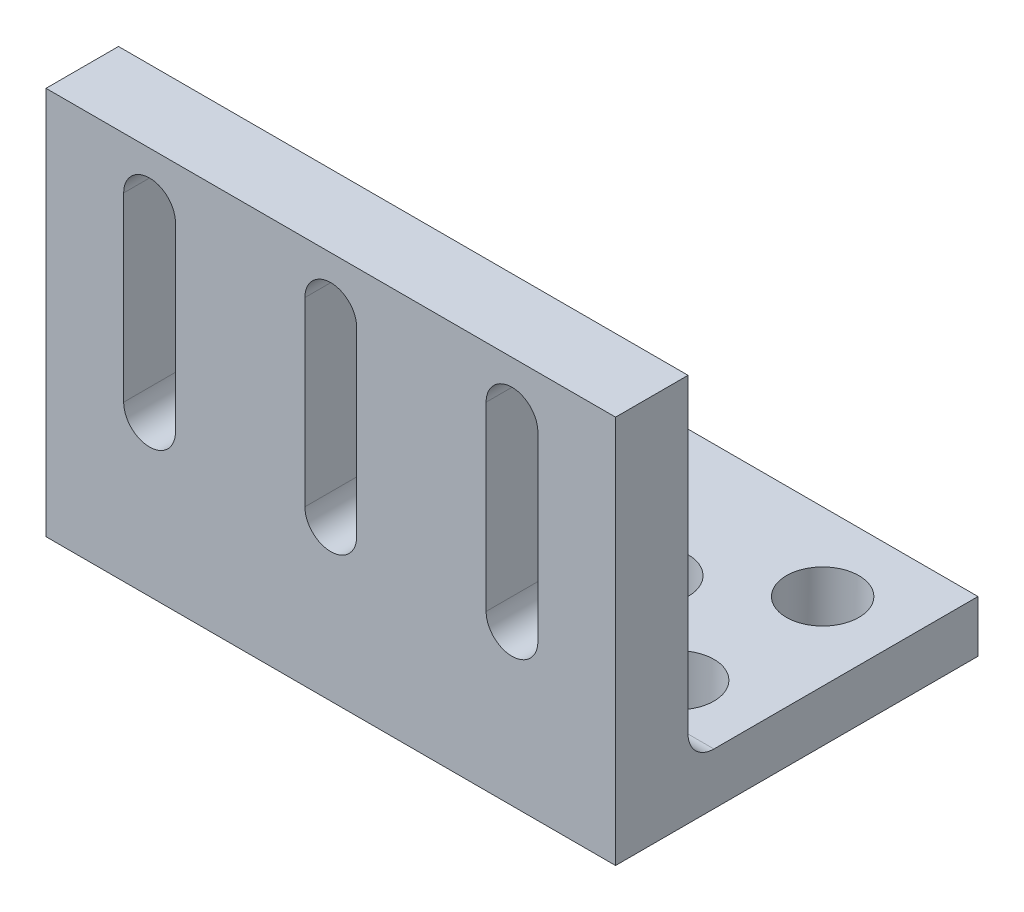
ISO-10303-21;
HEADER;
FILE_DESCRIPTION(('STEP AP214'),'2;1');
FILE_NAME('part.step','',(''),(''),'','','');
FILE_SCHEMA(('AUTOMOTIVE_DESIGN { 1 0 10303 214 1 1 1 1 }'));
ENDSEC;
DATA;
#1=APPLICATION_CONTEXT('core data for automotive mechanical design processes');
#2=APPLICATION_PROTOCOL_DEFINITION('international standard','automotive_design',2000,#1);
#3=PRODUCT_CONTEXT('',#1,'mechanical');
#4=PRODUCT('Part','Part','',(#3));
#5=PRODUCT_RELATED_PRODUCT_CATEGORY('part','',(#4));
#6=PRODUCT_DEFINITION_FORMATION('','',#4);
#7=PRODUCT_DEFINITION_CONTEXT('part definition',#1,'design');
#8=PRODUCT_DEFINITION('design','',#6,#7);
#9=PRODUCT_DEFINITION_SHAPE('','',#8);
#10=(LENGTH_UNIT() NAMED_UNIT(*) SI_UNIT(.MILLI.,.METRE.));
#11=(NAMED_UNIT(*) PLANE_ANGLE_UNIT() SI_UNIT($,.RADIAN.));
#12=(NAMED_UNIT(*) SI_UNIT($,.STERADIAN.) SOLID_ANGLE_UNIT());
#13=UNCERTAINTY_MEASURE_WITH_UNIT(LENGTH_MEASURE(1.E-05),#10,'distance_accuracy_value','');
#14=(GEOMETRIC_REPRESENTATION_CONTEXT(3) GLOBAL_UNCERTAINTY_ASSIGNED_CONTEXT((#13)) GLOBAL_UNIT_ASSIGNED_CONTEXT((#10,
#11,#12)) REPRESENTATION_CONTEXT('',''));
#15=CARTESIAN_POINT('',(0.,0.,0.));
#16=DIRECTION('',(0.,0.,1.));
#17=DIRECTION('',(1.,0.,0.));
#18=AXIS2_PLACEMENT_3D('',#15,#16,#17);
#19=CARTESIAN_POINT('',(-110.,0.,-70.));
#20=DIRECTION('',(0.,-1.,0.));
#21=DIRECTION('',(0.,0.,-1.));
#22=AXIS2_PLACEMENT_3D('',#19,#20,#21);
#23=PLANE('',#22);
#24=CARTESIAN_POINT('',(-75.,0.,-42.));
#25=DIRECTION('',(0.,-1.,0.));
#26=DIRECTION('',(0.,0.,-1.));
#27=AXIS2_PLACEMENT_3D('',#24,#25,#26);
#28=CIRCLE('',#27,7.00000000000001);
#29=CARTESIAN_POINT('',(-75.,0.,-35.));
#30=VERTEX_POINT('',#29);
#31=CARTESIAN_POINT('',(-75.,0.,-49.));
#32=VERTEX_POINT('',#31);
#33=EDGE_CURVE('E246',#30,#32,#28,.T.);
#34=ORIENTED_EDGE('',*,*,#33,.F.);
#35=DIRECTION('',(-1.,0.,0.));
#36=VECTOR('',#35,1.);
#37=CARTESIAN_POINT('',(-110.,0.,-35.));
#38=LINE('',#37,#36);
#39=CARTESIAN_POINT('',(-35.,0.,-35.));
#40=VERTEX_POINT('',#39);
#41=EDGE_CURVE('E243',#40,#30,#38,.T.);
#42=ORIENTED_EDGE('',*,*,#41,.F.);
#43=CARTESIAN_POINT('',(-35.,0.,-42.));
#44=DIRECTION('',(0.,-1.,0.));
#45=DIRECTION('',(0.,0.,-1.));
#46=AXIS2_PLACEMENT_3D('',#43,#44,#45);
#47=CIRCLE('',#46,7.);
#48=CARTESIAN_POINT('',(-35.,0.,-49.));
#49=VERTEX_POINT('',#48);
#50=EDGE_CURVE('E199',#49,#40,#47,.T.);
#51=ORIENTED_EDGE('',*,*,#50,.F.);
#52=DIRECTION('',(1.,0.,0.));
#53=VECTOR('',#52,1.);
#54=CARTESIAN_POINT('',(-110.,0.,-49.));
#55=LINE('',#54,#53);
#56=EDGE_CURVE('E249',#32,#49,#55,.T.);
#57=ORIENTED_EDGE('',*,*,#56,.F.);
#58=EDGE_LOOP('',(#34,#42,#51,#57));
#59=FACE_BOUND('',#58,.T.);
#60=CARTESIAN_POINT('',(-95.,0.,-27.));
#61=DIRECTION('',(0.,-1.,0.));
#62=DIRECTION('',(0.,0.,-1.));
#63=AXIS2_PLACEMENT_3D('',#60,#61,#62);
#64=CIRCLE('',#63,7.);
#65=CARTESIAN_POINT('',(-95.,0.,-34.));
#66=VERTEX_POINT('',#65);
#67=EDGE_CURVE('E241',#66,#66,#64,.T.);
#68=ORIENTED_EDGE('',*,*,#67,.F.);
#69=EDGE_LOOP('',(#68));
#70=FACE_BOUND('',#69,.T.);
#71=CARTESIAN_POINT('',(-15.,0.,-27.));
#72=DIRECTION('',(0.,-1.,0.));
#73=DIRECTION('',(0.,0.,-1.));
#74=AXIS2_PLACEMENT_3D('',#71,#72,#73);
#75=CIRCLE('',#74,7.);
#76=CARTESIAN_POINT('',(-15.,0.,-34.));
#77=VERTEX_POINT('',#76);
#78=EDGE_CURVE('E236',#77,#77,#75,.T.);
#79=ORIENTED_EDGE('',*,*,#78,.F.);
#80=EDGE_LOOP('',(#79));
#81=FACE_BOUND('',#80,.T.);
#82=CARTESIAN_POINT('',(-15.,0.,-55.));
#83=DIRECTION('',(0.,-1.,0.));
#84=DIRECTION('',(0.,0.,-1.));
#85=AXIS2_PLACEMENT_3D('',#82,#83,#84);
#86=CIRCLE('',#85,7.);
#87=CARTESIAN_POINT('',(-15.,0.,-62.));
#88=VERTEX_POINT('',#87);
#89=EDGE_CURVE('E233',#88,#88,#86,.T.);
#90=ORIENTED_EDGE('',*,*,#89,.F.);
#91=EDGE_LOOP('',(#90));
#92=FACE_BOUND('',#91,.T.);
#93=CARTESIAN_POINT('',(-95.,0.,-55.));
#94=DIRECTION('',(0.,-1.,0.));
#95=DIRECTION('',(0.,0.,-1.));
#96=AXIS2_PLACEMENT_3D('',#93,#94,#95);
#97=CIRCLE('',#96,7.);
#98=CARTESIAN_POINT('',(-95.,0.,-62.));
#99=VERTEX_POINT('',#98);
#100=EDGE_CURVE('E232',#99,#99,#97,.T.);
#101=ORIENTED_EDGE('',*,*,#100,.F.);
#102=EDGE_LOOP('',(#101));
#103=FACE_BOUND('',#102,.T.);
#104=DIRECTION('',(0.,0.,-1.));
#105=VECTOR('',#104,1.);
#106=CARTESIAN_POINT('',(0.,0.,-70.));
#107=LINE('',#106,#105);
#108=CARTESIAN_POINT('',(0.,0.,0.));
#109=VERTEX_POINT('',#108);
#110=CARTESIAN_POINT('',(0.,0.,-70.));
#111=VERTEX_POINT('',#110);
#112=EDGE_CURVE('E339',#109,#111,#107,.T.);
#113=ORIENTED_EDGE('',*,*,#112,.F.);
#114=DIRECTION('',(1.,0.,0.));
#115=VECTOR('',#114,1.);
#116=CARTESIAN_POINT('',(-110.,0.,0.));
#117=LINE('',#116,#115);
#118=CARTESIAN_POINT('',(-110.,0.,0.));
#119=VERTEX_POINT('',#118);
#120=EDGE_CURVE('E375',#119,#109,#117,.T.);
#121=ORIENTED_EDGE('',*,*,#120,.F.);
#122=DIRECTION('',(0.,0.,-1.));
#123=VECTOR('',#122,1.);
#124=CARTESIAN_POINT('',(-110.,0.,-70.));
#125=LINE('',#124,#123);
#126=CARTESIAN_POINT('',(-110.,0.,-70.));
#127=VERTEX_POINT('',#126);
#128=EDGE_CURVE('E338',#119,#127,#125,.T.);
#129=ORIENTED_EDGE('',*,*,#128,.T.);
#130=DIRECTION('',(1.,0.,0.));
#131=VECTOR('',#130,1.);
#132=CARTESIAN_POINT('',(-110.,0.,-70.));
#133=LINE('',#132,#131);
#134=EDGE_CURVE('E359',#127,#111,#133,.T.);
#135=ORIENTED_EDGE('',*,*,#134,.T.);
#136=EDGE_LOOP('',(#113,#121,#129,#135));
#137=FACE_BOUND('',#136,.T.);
#138=ADVANCED_FACE('F39',(#59,#70,#81,#92,#103,#137),#23,.T.);
#139=CARTESIAN_POINT('',(-110.,0.,0.));
#140=DIRECTION('',(0.,0.,1.));
#141=DIRECTION('',(1.,0.,0.));
#142=AXIS2_PLACEMENT_3D('',#139,#140,#141);
#143=PLANE('',#142);
#144=CARTESIAN_POINT('',(-20.,65.,0.));
#145=DIRECTION('',(0.,0.,1.));
#146=DIRECTION('',(1.,0.,0.));
#147=AXIS2_PLACEMENT_3D('',#144,#145,#146);
#148=CIRCLE('',#147,5.);
#149=CARTESIAN_POINT('',(-15.,65.,0.));
#150=VERTEX_POINT('',#149);
#151=CARTESIAN_POINT('',(-25.,65.,0.));
#152=VERTEX_POINT('',#151);
#153=EDGE_CURVE('E336',#150,#152,#148,.T.);
#154=ORIENTED_EDGE('',*,*,#153,.F.);
#155=DIRECTION('',(0.,1.,0.));
#156=VECTOR('',#155,1.);
#157=CARTESIAN_POINT('',(-15.,0.,0.));
#158=LINE('',#157,#156);
#159=CARTESIAN_POINT('',(-15.,30.,0.));
#160=VERTEX_POINT('',#159);
#161=EDGE_CURVE('E328',#160,#150,#158,.T.);
#162=ORIENTED_EDGE('',*,*,#161,.F.);
#163=CARTESIAN_POINT('',(-20.,30.,0.));
#164=DIRECTION('',(0.,0.,1.));
#165=DIRECTION('',(1.,0.,0.));
#166=AXIS2_PLACEMENT_3D('',#163,#164,#165);
#167=CIRCLE('',#166,5.);
#168=CARTESIAN_POINT('',(-25.,30.,0.));
#169=VERTEX_POINT('',#168);
#170=EDGE_CURVE('E332',#169,#160,#167,.T.);
#171=ORIENTED_EDGE('',*,*,#170,.F.);
#172=DIRECTION('',(0.,-1.,0.));
#173=VECTOR('',#172,1.);
#174=CARTESIAN_POINT('',(-25.,0.,0.));
#175=LINE('',#174,#173);
#176=EDGE_CURVE('E331',#152,#169,#175,.T.);
#177=ORIENTED_EDGE('',*,*,#176,.F.);
#178=EDGE_LOOP('',(#154,#162,#171,#177));
#179=FACE_BOUND('',#178,.T.);
#180=CARTESIAN_POINT('',(-55.,65.,0.));
#181=DIRECTION('',(0.,0.,1.));
#182=DIRECTION('',(1.,0.,0.));
#183=AXIS2_PLACEMENT_3D('',#180,#181,#182);
#184=CIRCLE('',#183,5.);
#185=CARTESIAN_POINT('',(-50.,65.,0.));
#186=VERTEX_POINT('',#185);
#187=CARTESIAN_POINT('',(-60.,65.,0.));
#188=VERTEX_POINT('',#187);
#189=EDGE_CURVE('E330',#186,#188,#184,.T.);
#190=ORIENTED_EDGE('',*,*,#189,.F.);
#191=DIRECTION('',(0.,1.,0.));
#192=VECTOR('',#191,1.);
#193=CARTESIAN_POINT('',(-50.,0.,0.));
#194=LINE('',#193,#192);
#195=CARTESIAN_POINT('',(-50.,30.,0.));
#196=VERTEX_POINT('',#195);
#197=EDGE_CURVE('E319',#196,#186,#194,.T.);
#198=ORIENTED_EDGE('',*,*,#197,.F.);
#199=CARTESIAN_POINT('',(-55.,30.,0.));
#200=DIRECTION('',(0.,0.,1.));
#201=DIRECTION('',(1.,0.,0.));
#202=AXIS2_PLACEMENT_3D('',#199,#200,#201);
#203=CIRCLE('',#202,5.);
#204=CARTESIAN_POINT('',(-60.,30.,0.));
#205=VERTEX_POINT('',#204);
#206=EDGE_CURVE('E325',#205,#196,#203,.T.);
#207=ORIENTED_EDGE('',*,*,#206,.F.);
#208=DIRECTION('',(0.,-1.,0.));
#209=VECTOR('',#208,1.);
#210=CARTESIAN_POINT('',(-60.,0.,0.));
#211=LINE('',#210,#209);
#212=EDGE_CURVE('E324',#188,#205,#211,.T.);
#213=ORIENTED_EDGE('',*,*,#212,.F.);
#214=EDGE_LOOP('',(#190,#198,#207,#213));
#215=FACE_BOUND('',#214,.T.);
#216=CARTESIAN_POINT('',(-90.,65.,0.));
#217=DIRECTION('',(0.,0.,1.));
#218=DIRECTION('',(1.,0.,0.));
#219=AXIS2_PLACEMENT_3D('',#216,#217,#218);
#220=CIRCLE('',#219,5.00000000000002);
#221=CARTESIAN_POINT('',(-85.,65.,0.));
#222=VERTEX_POINT('',#221);
#223=CARTESIAN_POINT('',(-95.,65.,0.));
#224=VERTEX_POINT('',#223);
#225=EDGE_CURVE('E318',#222,#224,#220,.T.);
#226=ORIENTED_EDGE('',*,*,#225,.F.);
#227=DIRECTION('',(0.,1.,0.));
#228=VECTOR('',#227,1.);
#229=CARTESIAN_POINT('',(-85.,0.,0.));
#230=LINE('',#229,#228);
#231=CARTESIAN_POINT('',(-85.,30.,0.));
#232=VERTEX_POINT('',#231);
#233=EDGE_CURVE('E270',#232,#222,#230,.T.);
#234=ORIENTED_EDGE('',*,*,#233,.F.);
#235=CARTESIAN_POINT('',(-90.,30.,0.));
#236=DIRECTION('',(0.,0.,1.));
#237=DIRECTION('',(1.,0.,0.));
#238=AXIS2_PLACEMENT_3D('',#235,#236,#237);
#239=CIRCLE('',#238,5.);
#240=CARTESIAN_POINT('',(-95.,30.,0.));
#241=VERTEX_POINT('',#240);
#242=EDGE_CURVE('E311',#241,#232,#239,.T.);
#243=ORIENTED_EDGE('',*,*,#242,.F.);
#244=DIRECTION('',(0.,-1.,0.));
#245=VECTOR('',#244,1.);
#246=CARTESIAN_POINT('',(-94.9999999999999,0.,0.));
#247=LINE('',#246,#245);
#248=EDGE_CURVE('E316',#224,#241,#247,.T.);
#249=ORIENTED_EDGE('',*,*,#248,.F.);
#250=EDGE_LOOP('',(#226,#234,#243,#249));
#251=FACE_BOUND('',#250,.T.);
#252=DIRECTION('',(0.,-1.,0.));
#253=VECTOR('',#252,1.);
#254=CARTESIAN_POINT('',(0.,0.,0.));
#255=LINE('',#254,#253);
#256=CARTESIAN_POINT('',(0.,75.,0.));
#257=VERTEX_POINT('',#256);
#258=EDGE_CURVE('E345',#257,#109,#255,.T.);
#259=ORIENTED_EDGE('',*,*,#258,.F.);
#260=DIRECTION('',(1.,0.,0.));
#261=VECTOR('',#260,1.);
#262=CARTESIAN_POINT('',(-110.,75.,0.));
#263=LINE('',#262,#261);
#264=CARTESIAN_POINT('',(-110.,75.,0.));
#265=VERTEX_POINT('',#264);
#266=EDGE_CURVE('E374',#265,#257,#263,.T.);
#267=ORIENTED_EDGE('',*,*,#266,.F.);
#268=DIRECTION('',(0.,-1.,0.));
#269=VECTOR('',#268,1.);
#270=CARTESIAN_POINT('',(-110.,0.,0.));
#271=LINE('',#270,#269);
#272=EDGE_CURVE('E353',#265,#119,#271,.T.);
#273=ORIENTED_EDGE('',*,*,#272,.T.);
#274=ORIENTED_EDGE('',*,*,#120,.T.);
#275=EDGE_LOOP('',(#259,#267,#273,#274));
#276=FACE_BOUND('',#275,.T.);
#277=ADVANCED_FACE('F409',(#179,#215,#251,#276),#143,.T.);
#278=CARTESIAN_POINT('',(-110.,75.,0.));
#279=DIRECTION('',(0.,1.,0.));
#280=DIRECTION('',(0.,0.,1.));
#281=AXIS2_PLACEMENT_3D('',#278,#279,#280);
#282=PLANE('',#281);
#283=DIRECTION('',(0.,0.,1.));
#284=VECTOR('',#283,1.);
#285=CARTESIAN_POINT('',(0.,75.,0.));
#286=LINE('',#285,#284);
#287=CARTESIAN_POINT('',(0.,75.,-14.));
#288=VERTEX_POINT('',#287);
#289=EDGE_CURVE('E370',#288,#257,#286,.T.);
#290=ORIENTED_EDGE('',*,*,#289,.F.);
#291=DIRECTION('',(1.,0.,0.));
#292=VECTOR('',#291,1.);
#293=CARTESIAN_POINT('',(-110.,75.,-14.));
#294=LINE('',#293,#292);
#295=CARTESIAN_POINT('',(-110.,75.,-14.));
#296=VERTEX_POINT('',#295);
#297=EDGE_CURVE('E380',#296,#288,#294,.T.);
#298=ORIENTED_EDGE('',*,*,#297,.F.);
#299=DIRECTION('',(0.,0.,1.));
#300=VECTOR('',#299,1.);
#301=CARTESIAN_POINT('',(-110.,75.,0.));
#302=LINE('',#301,#300);
#303=EDGE_CURVE('E351',#296,#265,#302,.T.);
#304=ORIENTED_EDGE('',*,*,#303,.T.);
#305=ORIENTED_EDGE('',*,*,#266,.T.);
#306=EDGE_LOOP('',(#290,#298,#304,#305));
#307=FACE_BOUND('',#306,.T.);
#308=ADVANCED_FACE('F413',(#307),#282,.T.);
#309=CARTESIAN_POINT('',(-110.,75.,-14.));
#310=DIRECTION('',(0.,0.,-1.));
#311=DIRECTION('',(0.,1.,0.));
#312=AXIS2_PLACEMENT_3D('',#309,#310,#311);
#313=PLANE('',#312);
#314=CARTESIAN_POINT('',(-20.,65.,-14.));
#315=DIRECTION('',(0.,0.,-1.));
#316=DIRECTION('',(0.,1.,0.));
#317=AXIS2_PLACEMENT_3D('',#314,#315,#316);
#318=CIRCLE('',#317,5.);
#319=CARTESIAN_POINT('',(-25.,65.,-14.));
#320=VERTEX_POINT('',#319);
#321=CARTESIAN_POINT('',(-15.,65.,-14.));
#322=VERTEX_POINT('',#321);
#323=EDGE_CURVE('E252',#320,#322,#318,.T.);
#324=ORIENTED_EDGE('',*,*,#323,.F.);
#325=DIRECTION('',(0.,1.,0.));
#326=VECTOR('',#325,1.);
#327=CARTESIAN_POINT('',(-25.,30.,-14.));
#328=LINE('',#327,#326);
#329=CARTESIAN_POINT('',(-25.,30.,-14.));
#330=VERTEX_POINT('',#329);
#331=EDGE_CURVE('E261',#330,#320,#328,.T.);
#332=ORIENTED_EDGE('',*,*,#331,.F.);
#333=CARTESIAN_POINT('',(-20.,30.,-14.));
#334=DIRECTION('',(0.,0.,-1.));
#335=DIRECTION('',(0.,1.,0.));
#336=AXIS2_PLACEMENT_3D('',#333,#334,#335);
#337=CIRCLE('',#336,5.);
#338=CARTESIAN_POINT('',(-15.,30.,-14.));
#339=VERTEX_POINT('',#338);
#340=EDGE_CURVE('E256',#339,#330,#337,.T.);
#341=ORIENTED_EDGE('',*,*,#340,.F.);
#342=DIRECTION('',(0.,-1.,0.));
#343=VECTOR('',#342,1.);
#344=CARTESIAN_POINT('',(-15.,65.,-14.));
#345=LINE('',#344,#343);
#346=EDGE_CURVE('E255',#322,#339,#345,.T.);
#347=ORIENTED_EDGE('',*,*,#346,.F.);
#348=EDGE_LOOP('',(#324,#332,#341,#347));
#349=FACE_BOUND('',#348,.T.);
#350=CARTESIAN_POINT('',(-55.,65.,-14.));
#351=DIRECTION('',(0.,0.,-1.));
#352=DIRECTION('',(0.,1.,0.));
#353=AXIS2_PLACEMENT_3D('',#350,#351,#352);
#354=CIRCLE('',#353,5.);
#355=CARTESIAN_POINT('',(-60.,65.,-14.));
#356=VERTEX_POINT('',#355);
#357=CARTESIAN_POINT('',(-50.,65.,-14.));
#358=VERTEX_POINT('',#357);
#359=EDGE_CURVE('E273',#356,#358,#354,.T.);
#360=ORIENTED_EDGE('',*,*,#359,.F.);
#361=DIRECTION('',(0.,1.,0.));
#362=VECTOR('',#361,1.);
#363=CARTESIAN_POINT('',(-60.,30.,-14.));
#364=LINE('',#363,#362);
#365=CARTESIAN_POINT('',(-60.,30.,-14.));
#366=VERTEX_POINT('',#365);
#367=EDGE_CURVE('E284',#366,#356,#364,.T.);
#368=ORIENTED_EDGE('',*,*,#367,.F.);
#369=CARTESIAN_POINT('',(-55.,30.,-14.));
#370=DIRECTION('',(0.,0.,-1.));
#371=DIRECTION('',(0.,1.,0.));
#372=AXIS2_PLACEMENT_3D('',#369,#370,#371);
#373=CIRCLE('',#372,5.);
#374=CARTESIAN_POINT('',(-50.,30.,-14.));
#375=VERTEX_POINT('',#374);
#376=EDGE_CURVE('E278',#375,#366,#373,.T.);
#377=ORIENTED_EDGE('',*,*,#376,.F.);
#378=DIRECTION('',(0.,-1.,0.));
#379=VECTOR('',#378,1.);
#380=CARTESIAN_POINT('',(-50.,65.,-14.));
#381=LINE('',#380,#379);
#382=EDGE_CURVE('E277',#358,#375,#381,.T.);
#383=ORIENTED_EDGE('',*,*,#382,.F.);
#384=EDGE_LOOP('',(#360,#368,#377,#383));
#385=FACE_BOUND('',#384,.T.);
#386=CARTESIAN_POINT('',(-90.,65.,-14.));
#387=DIRECTION('',(0.,0.,-1.));
#388=DIRECTION('',(0.,1.,0.));
#389=AXIS2_PLACEMENT_3D('',#386,#387,#388);
#390=CIRCLE('',#389,5.00000000000002);
#391=CARTESIAN_POINT('',(-95.,65.,-14.));
#392=VERTEX_POINT('',#391);
#393=CARTESIAN_POINT('',(-85.,65.,-14.));
#394=VERTEX_POINT('',#393);
#395=EDGE_CURVE('E253',#392,#394,#390,.T.);
#396=ORIENTED_EDGE('',*,*,#395,.F.);
#397=DIRECTION('',(0.,1.,0.));
#398=VECTOR('',#397,1.);
#399=CARTESIAN_POINT('',(-95.,30.,-14.));
#400=LINE('',#399,#398);
#401=CARTESIAN_POINT('',(-95.,30.,-14.));
#402=VERTEX_POINT('',#401);
#403=EDGE_CURVE('E302',#402,#392,#400,.T.);
#404=ORIENTED_EDGE('',*,*,#403,.F.);
#405=CARTESIAN_POINT('',(-90.,30.,-14.));
#406=DIRECTION('',(0.,0.,-1.));
#407=DIRECTION('',(0.,1.,0.));
#408=AXIS2_PLACEMENT_3D('',#405,#406,#407);
#409=CIRCLE('',#408,5.);
#410=CARTESIAN_POINT('',(-85.,30.,-14.));
#411=VERTEX_POINT('',#410);
#412=EDGE_CURVE('E299',#411,#402,#409,.T.);
#413=ORIENTED_EDGE('',*,*,#412,.F.);
#414=DIRECTION('',(0.,-1.,0.));
#415=VECTOR('',#414,1.);
#416=CARTESIAN_POINT('',(-85.,65.,-14.));
#417=LINE('',#416,#415);
#418=EDGE_CURVE('E293',#394,#411,#417,.T.);
#419=ORIENTED_EDGE('',*,*,#418,.F.);
#420=EDGE_LOOP('',(#396,#404,#413,#419));
#421=FACE_BOUND('',#420,.T.);
#422=DIRECTION('',(0.,1.,0.));
#423=VECTOR('',#422,1.);
#424=CARTESIAN_POINT('',(0.,75.,-14.));
#425=LINE('',#424,#423);
#426=CARTESIAN_POINT('',(0.,15.,-14.));
#427=VERTEX_POINT('',#426);
#428=EDGE_CURVE('E364',#427,#288,#425,.T.);
#429=ORIENTED_EDGE('',*,*,#428,.F.);
#430=DIRECTION('',(1.,0.,0.));
#431=VECTOR('',#430,1.);
#432=CARTESIAN_POINT('',(-110.,15.,-14.));
#433=LINE('',#432,#431);
#434=CARTESIAN_POINT('',(-110.,15.,-14.));
#435=VERTEX_POINT('',#434);
#436=EDGE_CURVE('E53',#427,#435,#433,.F.);
#437=ORIENTED_EDGE('',*,*,#436,.T.);
#438=DIRECTION('',(0.,1.,0.));
#439=VECTOR('',#438,1.);
#440=CARTESIAN_POINT('',(-110.,75.,-14.));
#441=LINE('',#440,#439);
#442=EDGE_CURVE('E349',#435,#296,#441,.T.);
#443=ORIENTED_EDGE('',*,*,#442,.T.);
#444=ORIENTED_EDGE('',*,*,#297,.T.);
#445=EDGE_LOOP('',(#429,#437,#443,#444));
#446=FACE_BOUND('',#445,.T.);
#447=ADVANCED_FACE('F422',(#349,#385,#421,#446),#313,.T.);
#448=CARTESIAN_POINT('',(-110.,10.,-14.));
#449=DIRECTION('',(0.,1.,0.));
#450=DIRECTION('',(0.,0.,1.));
#451=AXIS2_PLACEMENT_3D('',#448,#449,#450);
#452=PLANE('',#451);
#453=CARTESIAN_POINT('',(-75.,10.,-42.));
#454=DIRECTION('',(0.,1.,0.));
#455=DIRECTION('',(0.,0.,-1.));
#456=AXIS2_PLACEMENT_3D('',#453,#454,#455);
#457=CIRCLE('',#456,7.00000000000001);
#458=CARTESIAN_POINT('',(-75.,10.,-49.));
#459=VERTEX_POINT('',#458);
#460=CARTESIAN_POINT('',(-75.,10.,-35.));
#461=VERTEX_POINT('',#460);
#462=EDGE_CURVE('E213',#459,#461,#457,.T.);
#463=ORIENTED_EDGE('',*,*,#462,.F.);
#464=DIRECTION('',(-1.,0.,0.));
#465=VECTOR('',#464,1.);
#466=CARTESIAN_POINT('',(-75.,10.,-49.));
#467=LINE('',#466,#465);
#468=CARTESIAN_POINT('',(-35.,10.,-49.));
#469=VERTEX_POINT('',#468);
#470=EDGE_CURVE('E217',#469,#459,#467,.T.);
#471=ORIENTED_EDGE('',*,*,#470,.F.);
#472=CARTESIAN_POINT('',(-35.,10.,-42.));
#473=DIRECTION('',(0.,1.,0.));
#474=DIRECTION('',(0.,0.,-1.));
#475=AXIS2_PLACEMENT_3D('',#472,#473,#474);
#476=CIRCLE('',#475,7.);
#477=CARTESIAN_POINT('',(-35.,10.,-35.));
#478=VERTEX_POINT('',#477);
#479=EDGE_CURVE('E197',#478,#469,#476,.T.);
#480=ORIENTED_EDGE('',*,*,#479,.F.);
#481=DIRECTION('',(1.,0.,0.));
#482=VECTOR('',#481,1.);
#483=CARTESIAN_POINT('',(-35.,10.,-35.));
#484=LINE('',#483,#482);
#485=EDGE_CURVE('E208',#461,#478,#484,.T.);
#486=ORIENTED_EDGE('',*,*,#485,.F.);
#487=EDGE_LOOP('',(#463,#471,#480,#486));
#488=FACE_BOUND('',#487,.T.);
#489=CARTESIAN_POINT('',(-95.,10.,-27.));
#490=DIRECTION('',(0.,1.,0.));
#491=DIRECTION('',(0.,0.,1.));
#492=AXIS2_PLACEMENT_3D('',#489,#490,#491);
#493=CIRCLE('',#492,7.);
#494=CARTESIAN_POINT('',(-95.,10.,-20.));
#495=VERTEX_POINT('',#494);
#496=EDGE_CURVE('E223',#495,#495,#493,.T.);
#497=ORIENTED_EDGE('',*,*,#496,.F.);
#498=EDGE_LOOP('',(#497));
#499=FACE_BOUND('',#498,.T.);
#500=CARTESIAN_POINT('',(-15.,10.,-27.));
#501=DIRECTION('',(0.,1.,0.));
#502=DIRECTION('',(0.,0.,1.));
#503=AXIS2_PLACEMENT_3D('',#500,#501,#502);
#504=CIRCLE('',#503,7.);
#505=CARTESIAN_POINT('',(-15.,10.,-20.));
#506=VERTEX_POINT('',#505);
#507=EDGE_CURVE('E511',#506,#506,#504,.T.);
#508=ORIENTED_EDGE('',*,*,#507,.F.);
#509=EDGE_LOOP('',(#508));
#510=FACE_BOUND('',#509,.T.);
#511=CARTESIAN_POINT('',(-15.,10.,-55.));
#512=DIRECTION('',(0.,1.,0.));
#513=DIRECTION('',(0.,0.,1.));
#514=AXIS2_PLACEMENT_3D('',#511,#512,#513);
#515=CIRCLE('',#514,7.);
#516=CARTESIAN_POINT('',(-15.,10.,-48.));
#517=VERTEX_POINT('',#516);
#518=EDGE_CURVE('E234',#517,#517,#515,.T.);
#519=ORIENTED_EDGE('',*,*,#518,.F.);
#520=EDGE_LOOP('',(#519));
#521=FACE_BOUND('',#520,.T.);
#522=CARTESIAN_POINT('',(-95.,10.,-55.));
#523=DIRECTION('',(0.,1.,0.));
#524=DIRECTION('',(0.,0.,1.));
#525=AXIS2_PLACEMENT_3D('',#522,#523,#524);
#526=CIRCLE('',#525,7.);
#527=CARTESIAN_POINT('',(-95.,10.,-48.));
#528=VERTEX_POINT('',#527);
#529=EDGE_CURVE('E229',#528,#528,#526,.T.);
#530=ORIENTED_EDGE('',*,*,#529,.F.);
#531=EDGE_LOOP('',(#530));
#532=FACE_BOUND('',#531,.T.);
#533=DIRECTION('',(0.,0.,1.));
#534=VECTOR('',#533,1.);
#535=CARTESIAN_POINT('',(-110.,10.,-14.));
#536=LINE('',#535,#534);
#537=CARTESIAN_POINT('',(-110.,10.,-70.));
#538=VERTEX_POINT('',#537);
#539=CARTESIAN_POINT('',(-110.,10.,-19.));
#540=VERTEX_POINT('',#539);
#541=EDGE_CURVE('E347',#538,#540,#536,.T.);
#542=ORIENTED_EDGE('',*,*,#541,.T.);
#543=DIRECTION('',(1.,0.,0.));
#544=VECTOR('',#543,1.);
#545=CARTESIAN_POINT('',(0.,10.,-19.));
#546=LINE('',#545,#544);
#547=CARTESIAN_POINT('',(0.,10.,-19.));
#548=VERTEX_POINT('',#547);
#549=EDGE_CURVE('E372',#540,#548,#546,.T.);
#550=ORIENTED_EDGE('',*,*,#549,.T.);
#551=DIRECTION('',(0.,0.,1.));
#552=VECTOR('',#551,1.);
#553=CARTESIAN_POINT('',(0.,10.,-14.));
#554=LINE('',#553,#552);
#555=CARTESIAN_POINT('',(0.,10.,-70.));
#556=VERTEX_POINT('',#555);
#557=EDGE_CURVE('E361',#556,#548,#554,.T.);
#558=ORIENTED_EDGE('',*,*,#557,.F.);
#559=DIRECTION('',(1.,0.,0.));
#560=VECTOR('',#559,1.);
#561=CARTESIAN_POINT('',(-110.,10.,-70.));
#562=LINE('',#561,#560);
#563=EDGE_CURVE('E379',#538,#556,#562,.T.);
#564=ORIENTED_EDGE('',*,*,#563,.F.);
#565=EDGE_LOOP('',(#542,#550,#558,#564));
#566=FACE_BOUND('',#565,.T.);
#567=ADVANCED_FACE('F214',(#488,#499,#510,#521,#532,#566),#452,.T.);
#568=CARTESIAN_POINT('',(-110.,10.,-70.));
#569=DIRECTION('',(0.,0.,-1.));
#570=DIRECTION('',(-1.,0.,0.));
#571=AXIS2_PLACEMENT_3D('',#568,#569,#570);
#572=PLANE('',#571);
#573=DIRECTION('',(0.,1.,0.));
#574=VECTOR('',#573,1.);
#575=CARTESIAN_POINT('',(0.,10.,-70.));
#576=LINE('',#575,#574);
#577=EDGE_CURVE('E358',#111,#556,#576,.T.);
#578=ORIENTED_EDGE('',*,*,#577,.F.);
#579=ORIENTED_EDGE('',*,*,#134,.F.);
#580=DIRECTION('',(0.,1.,0.));
#581=VECTOR('',#580,1.);
#582=CARTESIAN_POINT('',(-110.,10.,-70.));
#583=LINE('',#582,#581);
#584=EDGE_CURVE('E344',#127,#538,#583,.T.);
#585=ORIENTED_EDGE('',*,*,#584,.T.);
#586=ORIENTED_EDGE('',*,*,#563,.T.);
#587=EDGE_LOOP('',(#578,#579,#585,#586));
#588=FACE_BOUND('',#587,.T.);
#589=ADVANCED_FACE('F395',(#588),#572,.T.);
#590=CARTESIAN_POINT('',(-110.,0.,0.));
#591=DIRECTION('',(-1.,0.,0.));
#592=DIRECTION('',(0.,0.,1.));
#593=AXIS2_PLACEMENT_3D('',#590,#591,#592);
#594=PLANE('',#593);
#595=ORIENTED_EDGE('',*,*,#128,.F.);
#596=ORIENTED_EDGE('',*,*,#272,.F.);
#597=ORIENTED_EDGE('',*,*,#303,.F.);
#598=ORIENTED_EDGE('',*,*,#442,.F.);
#599=CARTESIAN_POINT('',(-110.,15.,-19.));
#600=DIRECTION('',(-1.,0.,0.));
#601=DIRECTION('',(0.,0.,1.));
#602=AXIS2_PLACEMENT_3D('',#599,#600,#601);
#603=CIRCLE('',#602,5.);
#604=EDGE_CURVE('E11',#435,#540,#603,.F.);
#605=ORIENTED_EDGE('',*,*,#604,.T.);
#606=ORIENTED_EDGE('',*,*,#541,.F.);
#607=ORIENTED_EDGE('',*,*,#584,.F.);
#608=EDGE_LOOP('',(#595,#596,#597,#598,#605,#606,#607));
#609=FACE_BOUND('',#608,.T.);
#610=ADVANCED_FACE('F396',(#609),#594,.T.);
#611=CARTESIAN_POINT('',(0.,0.,0.));
#612=DIRECTION('',(-1.,0.,0.));
#613=DIRECTION('',(0.,0.,1.));
#614=AXIS2_PLACEMENT_3D('',#611,#612,#613);
#615=PLANE('',#614);
#616=ORIENTED_EDGE('',*,*,#112,.T.);
#617=ORIENTED_EDGE('',*,*,#577,.T.);
#618=ORIENTED_EDGE('',*,*,#557,.T.);
#619=CARTESIAN_POINT('',(0.,15.,-19.));
#620=DIRECTION('',(-1.,0.,0.));
#621=DIRECTION('',(0.,0.,1.));
#622=AXIS2_PLACEMENT_3D('',#619,#620,#621);
#623=CIRCLE('',#622,5.);
#624=EDGE_CURVE('E50',#548,#427,#623,.T.);
#625=ORIENTED_EDGE('',*,*,#624,.T.);
#626=ORIENTED_EDGE('',*,*,#428,.T.);
#627=ORIENTED_EDGE('',*,*,#289,.T.);
#628=ORIENTED_EDGE('',*,*,#258,.T.);
#629=EDGE_LOOP('',(#616,#617,#618,#625,#626,#627,#628));
#630=FACE_BOUND('',#629,.T.);
#631=ADVANCED_FACE('F391',(#630),#615,.F.);
#632=CARTESIAN_POINT('',(-90.,65.,96.));
#633=DIRECTION('',(0.,0.,-1.));
#634=DIRECTION('',(0.,1.,0.));
#635=AXIS2_PLACEMENT_3D('',#632,#633,#634);
#636=CYLINDRICAL_SURFACE('',#635,5.00000000000002);
#637=ORIENTED_EDGE('',*,*,#225,.T.);
#638=DIRECTION('',(0.,0.,-1.));
#639=VECTOR('',#638,1.);
#640=CARTESIAN_POINT('',(-95.,65.,96.));
#641=LINE('',#640,#639);
#642=EDGE_CURVE('E280',#224,#392,#641,.T.);
#643=ORIENTED_EDGE('',*,*,#642,.T.);
#644=ORIENTED_EDGE('',*,*,#395,.T.);
#645=DIRECTION('',(0.,0.,-1.));
#646=VECTOR('',#645,1.);
#647=CARTESIAN_POINT('',(-85.,65.,96.));
#648=LINE('',#647,#646);
#649=EDGE_CURVE('E301',#222,#394,#648,.T.);
#650=ORIENTED_EDGE('',*,*,#649,.F.);
#651=EDGE_LOOP('',(#637,#643,#644,#650));
#652=FACE_BOUND('',#651,.T.);
#653=ADVANCED_FACE('F433',(#652),#636,.F.);
#654=CARTESIAN_POINT('',(-95.,30.,96.));
#655=DIRECTION('',(-1.,0.,0.));
#656=DIRECTION('',(0.,-1.,0.));
#657=AXIS2_PLACEMENT_3D('',#654,#655,#656);
#658=PLANE('',#657);
#659=ORIENTED_EDGE('',*,*,#248,.T.);
#660=DIRECTION('',(0.,0.,-1.));
#661=VECTOR('',#660,1.);
#662=CARTESIAN_POINT('',(-95.,30.,96.));
#663=LINE('',#662,#661);
#664=EDGE_CURVE('E308',#241,#402,#663,.T.);
#665=ORIENTED_EDGE('',*,*,#664,.T.);
#666=ORIENTED_EDGE('',*,*,#403,.T.);
#667=ORIENTED_EDGE('',*,*,#642,.F.);
#668=EDGE_LOOP('',(#659,#665,#666,#667));
#669=FACE_BOUND('',#668,.T.);
#670=ADVANCED_FACE('F437',(#669),#658,.F.);
#671=CARTESIAN_POINT('',(-90.,30.,96.));
#672=DIRECTION('',(0.,0.,-1.));
#673=DIRECTION('',(0.,1.,0.));
#674=AXIS2_PLACEMENT_3D('',#671,#672,#673);
#675=CYLINDRICAL_SURFACE('',#674,5.);
#676=ORIENTED_EDGE('',*,*,#242,.T.);
#677=DIRECTION('',(0.,0.,-1.));
#678=VECTOR('',#677,1.);
#679=CARTESIAN_POINT('',(-85.,30.,96.));
#680=LINE('',#679,#678);
#681=EDGE_CURVE('E306',#232,#411,#680,.T.);
#682=ORIENTED_EDGE('',*,*,#681,.T.);
#683=ORIENTED_EDGE('',*,*,#412,.T.);
#684=ORIENTED_EDGE('',*,*,#664,.F.);
#685=EDGE_LOOP('',(#676,#682,#683,#684));
#686=FACE_BOUND('',#685,.T.);
#687=ADVANCED_FACE('F441',(#686),#675,.F.);
#688=CARTESIAN_POINT('',(-85.,65.,96.));
#689=DIRECTION('',(1.,0.,0.));
#690=DIRECTION('',(0.,0.,-1.));
#691=AXIS2_PLACEMENT_3D('',#688,#689,#690);
#692=PLANE('',#691);
#693=ORIENTED_EDGE('',*,*,#233,.T.);
#694=ORIENTED_EDGE('',*,*,#649,.T.);
#695=ORIENTED_EDGE('',*,*,#418,.T.);
#696=ORIENTED_EDGE('',*,*,#681,.F.);
#697=EDGE_LOOP('',(#693,#694,#695,#696));
#698=FACE_BOUND('',#697,.T.);
#699=ADVANCED_FACE('F439',(#698),#692,.F.);
#700=CARTESIAN_POINT('',(-55.,65.,96.));
#701=DIRECTION('',(0.,0.,-1.));
#702=DIRECTION('',(0.,1.,0.));
#703=AXIS2_PLACEMENT_3D('',#700,#701,#702);
#704=CYLINDRICAL_SURFACE('',#703,5.);
#705=ORIENTED_EDGE('',*,*,#189,.T.);
#706=DIRECTION('',(0.,0.,-1.));
#707=VECTOR('',#706,1.);
#708=CARTESIAN_POINT('',(-60.,65.,96.));
#709=LINE('',#708,#707);
#710=EDGE_CURVE('E254',#188,#356,#709,.T.);
#711=ORIENTED_EDGE('',*,*,#710,.T.);
#712=ORIENTED_EDGE('',*,*,#359,.T.);
#713=DIRECTION('',(0.,0.,-1.));
#714=VECTOR('',#713,1.);
#715=CARTESIAN_POINT('',(-50.,65.,96.));
#716=LINE('',#715,#714);
#717=EDGE_CURVE('E287',#186,#358,#716,.T.);
#718=ORIENTED_EDGE('',*,*,#717,.F.);
#719=EDGE_LOOP('',(#705,#711,#712,#718));
#720=FACE_BOUND('',#719,.T.);
#721=ADVANCED_FACE('F444',(#720),#704,.F.);
#722=CARTESIAN_POINT('',(-60.,30.,96.));
#723=DIRECTION('',(-1.,0.,0.));
#724=DIRECTION('',(0.,-1.,0.));
#725=AXIS2_PLACEMENT_3D('',#722,#723,#724);
#726=PLANE('',#725);
#727=ORIENTED_EDGE('',*,*,#212,.T.);
#728=DIRECTION('',(0.,0.,-1.));
#729=VECTOR('',#728,1.);
#730=CARTESIAN_POINT('',(-60.,30.,96.));
#731=LINE('',#730,#729);
#732=EDGE_CURVE('E290',#205,#366,#731,.T.);
#733=ORIENTED_EDGE('',*,*,#732,.T.);
#734=ORIENTED_EDGE('',*,*,#367,.T.);
#735=ORIENTED_EDGE('',*,*,#710,.F.);
#736=EDGE_LOOP('',(#727,#733,#734,#735));
#737=FACE_BOUND('',#736,.T.);
#738=ADVANCED_FACE('F451',(#737),#726,.F.);
#739=CARTESIAN_POINT('',(-55.,30.,96.));
#740=DIRECTION('',(0.,0.,-1.));
#741=DIRECTION('',(0.,1.,0.));
#742=AXIS2_PLACEMENT_3D('',#739,#740,#741);
#743=CYLINDRICAL_SURFACE('',#742,5.);
#744=ORIENTED_EDGE('',*,*,#206,.T.);
#745=DIRECTION('',(0.,0.,-1.));
#746=VECTOR('',#745,1.);
#747=CARTESIAN_POINT('',(-50.,30.,96.));
#748=LINE('',#747,#746);
#749=EDGE_CURVE('E288',#196,#375,#748,.T.);
#750=ORIENTED_EDGE('',*,*,#749,.T.);
#751=ORIENTED_EDGE('',*,*,#376,.T.);
#752=ORIENTED_EDGE('',*,*,#732,.F.);
#753=EDGE_LOOP('',(#744,#750,#751,#752));
#754=FACE_BOUND('',#753,.T.);
#755=ADVANCED_FACE('F458',(#754),#743,.F.);
#756=CARTESIAN_POINT('',(-50.,65.,96.));
#757=DIRECTION('',(1.,0.,0.));
#758=DIRECTION('',(0.,1.,0.));
#759=AXIS2_PLACEMENT_3D('',#756,#757,#758);
#760=PLANE('',#759);
#761=ORIENTED_EDGE('',*,*,#197,.T.);
#762=ORIENTED_EDGE('',*,*,#717,.T.);
#763=ORIENTED_EDGE('',*,*,#382,.T.);
#764=ORIENTED_EDGE('',*,*,#749,.F.);
#765=EDGE_LOOP('',(#761,#762,#763,#764));
#766=FACE_BOUND('',#765,.T.);
#767=ADVANCED_FACE('F457',(#766),#760,.F.);
#768=CARTESIAN_POINT('',(-20.,65.,96.));
#769=DIRECTION('',(0.,0.,-1.));
#770=DIRECTION('',(0.,1.,0.));
#771=AXIS2_PLACEMENT_3D('',#768,#769,#770);
#772=CYLINDRICAL_SURFACE('',#771,5.);
#773=ORIENTED_EDGE('',*,*,#153,.T.);
#774=DIRECTION('',(0.,0.,-1.));
#775=VECTOR('',#774,1.);
#776=CARTESIAN_POINT('',(-25.,65.,96.));
#777=LINE('',#776,#775);
#778=EDGE_CURVE('E264',#152,#320,#777,.T.);
#779=ORIENTED_EDGE('',*,*,#778,.T.);
#780=ORIENTED_EDGE('',*,*,#323,.T.);
#781=DIRECTION('',(0.,0.,-1.));
#782=VECTOR('',#781,1.);
#783=CARTESIAN_POINT('',(-15.,65.,96.));
#784=LINE('',#783,#782);
#785=EDGE_CURVE('E262',#150,#322,#784,.T.);
#786=ORIENTED_EDGE('',*,*,#785,.F.);
#787=EDGE_LOOP('',(#773,#779,#780,#786));
#788=FACE_BOUND('',#787,.T.);
#789=ADVANCED_FACE('F459',(#788),#772,.F.);
#790=CARTESIAN_POINT('',(-25.,30.,96.));
#791=DIRECTION('',(-1.,0.,0.));
#792=DIRECTION('',(0.,0.,1.));
#793=AXIS2_PLACEMENT_3D('',#790,#791,#792);
#794=PLANE('',#793);
#795=ORIENTED_EDGE('',*,*,#176,.T.);
#796=DIRECTION('',(0.,0.,-1.));
#797=VECTOR('',#796,1.);
#798=CARTESIAN_POINT('',(-25.,30.,96.));
#799=LINE('',#798,#797);
#800=EDGE_CURVE('E268',#169,#330,#799,.T.);
#801=ORIENTED_EDGE('',*,*,#800,.T.);
#802=ORIENTED_EDGE('',*,*,#331,.T.);
#803=ORIENTED_EDGE('',*,*,#778,.F.);
#804=EDGE_LOOP('',(#795,#801,#802,#803));
#805=FACE_BOUND('',#804,.T.);
#806=ADVANCED_FACE('F468',(#805),#794,.F.);
#807=CARTESIAN_POINT('',(-20.,30.,96.));
#808=DIRECTION('',(0.,0.,-1.));
#809=DIRECTION('',(0.,1.,0.));
#810=AXIS2_PLACEMENT_3D('',#807,#808,#809);
#811=CYLINDRICAL_SURFACE('',#810,5.);
#812=ORIENTED_EDGE('',*,*,#170,.T.);
#813=DIRECTION('',(0.,0.,-1.));
#814=VECTOR('',#813,1.);
#815=CARTESIAN_POINT('',(-15.,30.,96.));
#816=LINE('',#815,#814);
#817=EDGE_CURVE('E269',#160,#339,#816,.T.);
#818=ORIENTED_EDGE('',*,*,#817,.T.);
#819=ORIENTED_EDGE('',*,*,#340,.T.);
#820=ORIENTED_EDGE('',*,*,#800,.F.);
#821=EDGE_LOOP('',(#812,#818,#819,#820));
#822=FACE_BOUND('',#821,.T.);
#823=ADVANCED_FACE('F474',(#822),#811,.F.);
#824=CARTESIAN_POINT('',(-15.,65.,96.));
#825=DIRECTION('',(1.,0.,0.));
#826=DIRECTION('',(0.,1.,0.));
#827=AXIS2_PLACEMENT_3D('',#824,#825,#826);
#828=PLANE('',#827);
#829=ORIENTED_EDGE('',*,*,#161,.T.);
#830=ORIENTED_EDGE('',*,*,#785,.T.);
#831=ORIENTED_EDGE('',*,*,#346,.T.);
#832=ORIENTED_EDGE('',*,*,#817,.F.);
#833=EDGE_LOOP('',(#829,#830,#831,#832));
#834=FACE_BOUND('',#833,.T.);
#835=ADVANCED_FACE('F472',(#834),#828,.F.);
#836=CARTESIAN_POINT('',(-95.,-100.,-55.));
#837=DIRECTION('',(0.,1.,0.));
#838=DIRECTION('',(0.,0.,1.));
#839=AXIS2_PLACEMENT_3D('',#836,#837,#838);
#840=CYLINDRICAL_SURFACE('',#839,7.);
#841=ORIENTED_EDGE('',*,*,#100,.T.);
#842=EDGE_LOOP('',(#841));
#843=FACE_BOUND('',#842,.T.);
#844=ORIENTED_EDGE('',*,*,#529,.T.);
#845=EDGE_LOOP('',(#844));
#846=FACE_BOUND('',#845,.T.);
#847=ADVANCED_FACE('F475',(#843,#846),#840,.F.);
#848=CARTESIAN_POINT('',(-15.,-100.,-55.));
#849=DIRECTION('',(0.,1.,0.));
#850=DIRECTION('',(0.,0.,1.));
#851=AXIS2_PLACEMENT_3D('',#848,#849,#850);
#852=CYLINDRICAL_SURFACE('',#851,7.);
#853=ORIENTED_EDGE('',*,*,#89,.T.);
#854=EDGE_LOOP('',(#853));
#855=FACE_BOUND('',#854,.T.);
#856=ORIENTED_EDGE('',*,*,#518,.T.);
#857=EDGE_LOOP('',(#856));
#858=FACE_BOUND('',#857,.T.);
#859=ADVANCED_FACE('F482',(#855,#858),#852,.F.);
#860=CARTESIAN_POINT('',(-15.,-100.,-27.));
#861=DIRECTION('',(0.,1.,0.));
#862=DIRECTION('',(0.,0.,1.));
#863=AXIS2_PLACEMENT_3D('',#860,#861,#862);
#864=CYLINDRICAL_SURFACE('',#863,7.);
#865=ORIENTED_EDGE('',*,*,#78,.T.);
#866=EDGE_LOOP('',(#865));
#867=FACE_BOUND('',#866,.T.);
#868=ORIENTED_EDGE('',*,*,#507,.T.);
#869=EDGE_LOOP('',(#868));
#870=FACE_BOUND('',#869,.T.);
#871=ADVANCED_FACE('F496',(#867,#870),#864,.F.);
#872=CARTESIAN_POINT('',(-95.,-100.,-27.));
#873=DIRECTION('',(0.,1.,0.));
#874=DIRECTION('',(0.,0.,1.));
#875=AXIS2_PLACEMENT_3D('',#872,#873,#874);
#876=CYLINDRICAL_SURFACE('',#875,7.);
#877=ORIENTED_EDGE('',*,*,#67,.T.);
#878=EDGE_LOOP('',(#877));
#879=FACE_BOUND('',#878,.T.);
#880=ORIENTED_EDGE('',*,*,#496,.T.);
#881=EDGE_LOOP('',(#880));
#882=FACE_BOUND('',#881,.T.);
#883=ADVANCED_FACE('F487',(#879,#882),#876,.F.);
#884=CARTESIAN_POINT('',(-75.,-100.,-42.));
#885=DIRECTION('',(0.,1.,0.));
#886=DIRECTION('',(0.,0.,1.));
#887=AXIS2_PLACEMENT_3D('',#884,#885,#886);
#888=CYLINDRICAL_SURFACE('',#887,7.00000000000001);
#889=ORIENTED_EDGE('',*,*,#33,.T.);
#890=DIRECTION('',(0.,1.,0.));
#891=VECTOR('',#890,1.);
#892=CARTESIAN_POINT('',(-75.,-100.,-49.));
#893=LINE('',#892,#891);
#894=EDGE_CURVE('E224',#32,#459,#893,.T.);
#895=ORIENTED_EDGE('',*,*,#894,.T.);
#896=ORIENTED_EDGE('',*,*,#462,.T.);
#897=DIRECTION('',(0.,1.,0.));
#898=VECTOR('',#897,1.);
#899=CARTESIAN_POINT('',(-75.,-100.,-35.));
#900=LINE('',#899,#898);
#901=EDGE_CURVE('E204',#30,#461,#900,.T.);
#902=ORIENTED_EDGE('',*,*,#901,.F.);
#903=EDGE_LOOP('',(#889,#895,#896,#902));
#904=FACE_BOUND('',#903,.T.);
#905=ADVANCED_FACE('F486',(#904),#888,.F.);
#906=CARTESIAN_POINT('',(-75.,-100.,-49.));
#907=DIRECTION('',(0.,0.,-1.));
#908=DIRECTION('',(-1.,0.,0.));
#909=AXIS2_PLACEMENT_3D('',#906,#907,#908);
#910=PLANE('',#909);
#911=ORIENTED_EDGE('',*,*,#56,.T.);
#912=DIRECTION('',(0.,1.,0.));
#913=VECTOR('',#912,1.);
#914=CARTESIAN_POINT('',(-35.,-100.,-49.));
#915=LINE('',#914,#913);
#916=EDGE_CURVE('E201',#49,#469,#915,.T.);
#917=ORIENTED_EDGE('',*,*,#916,.T.);
#918=ORIENTED_EDGE('',*,*,#470,.T.);
#919=ORIENTED_EDGE('',*,*,#894,.F.);
#920=EDGE_LOOP('',(#911,#917,#918,#919));
#921=FACE_BOUND('',#920,.T.);
#922=ADVANCED_FACE('F488',(#921),#910,.F.);
#923=CARTESIAN_POINT('',(-35.,-100.,-42.));
#924=DIRECTION('',(0.,1.,0.));
#925=DIRECTION('',(0.,0.,1.));
#926=AXIS2_PLACEMENT_3D('',#923,#924,#925);
#927=CYLINDRICAL_SURFACE('',#926,7.);
#928=ORIENTED_EDGE('',*,*,#50,.T.);
#929=DIRECTION('',(0.,1.,0.));
#930=VECTOR('',#929,1.);
#931=CARTESIAN_POINT('',(-35.,-100.,-35.));
#932=LINE('',#931,#930);
#933=EDGE_CURVE('E194',#40,#478,#932,.T.);
#934=ORIENTED_EDGE('',*,*,#933,.T.);
#935=ORIENTED_EDGE('',*,*,#479,.T.);
#936=ORIENTED_EDGE('',*,*,#916,.F.);
#937=EDGE_LOOP('',(#928,#934,#935,#936));
#938=FACE_BOUND('',#937,.T.);
#939=ADVANCED_FACE('F191',(#938),#927,.F.);
#940=CARTESIAN_POINT('',(-35.,-100.,-35.));
#941=DIRECTION('',(0.,0.,1.));
#942=DIRECTION('',(1.,0.,0.));
#943=AXIS2_PLACEMENT_3D('',#940,#941,#942);
#944=PLANE('',#943);
#945=ORIENTED_EDGE('',*,*,#41,.T.);
#946=ORIENTED_EDGE('',*,*,#901,.T.);
#947=ORIENTED_EDGE('',*,*,#485,.T.);
#948=ORIENTED_EDGE('',*,*,#933,.F.);
#949=EDGE_LOOP('',(#945,#946,#947,#948));
#950=FACE_BOUND('',#949,.T.);
#951=ADVANCED_FACE('F207',(#950),#944,.F.);
#952=CARTESIAN_POINT('',(-110.,15.,-19.));
#953=DIRECTION('',(-1.,0.,0.));
#954=DIRECTION('',(0.,0.,1.));
#955=AXIS2_PLACEMENT_3D('',#952,#953,#954);
#956=CYLINDRICAL_SURFACE('',#955,5.);
#957=ORIENTED_EDGE('',*,*,#604,.F.);
#958=ORIENTED_EDGE('',*,*,#436,.F.);
#959=ORIENTED_EDGE('',*,*,#624,.F.);
#960=ORIENTED_EDGE('',*,*,#549,.F.);
#961=EDGE_LOOP('',(#957,#958,#959,#960));
#962=FACE_BOUND('',#961,.T.);
#963=ADVANCED_FACE('F41',(#962),#956,.F.);
#964=CLOSED_SHELL('',(#138,#277,#308,#447,#567,#589,#610,#631,#653,#670,#687,#699,#721,#738,
#755,#767,#789,#806,#823,#835,#847,#859,#871,#883,#905,#922,#939,#951,#963));
#965=MANIFOLD_SOLID_BREP('B2',#964);
#966=ADVANCED_BREP_SHAPE_REPRESENTATION('',(#18,#965),#14);
#967=SHAPE_DEFINITION_REPRESENTATION(#9,#966);
ENDSEC;
END-ISO-10303-21;
